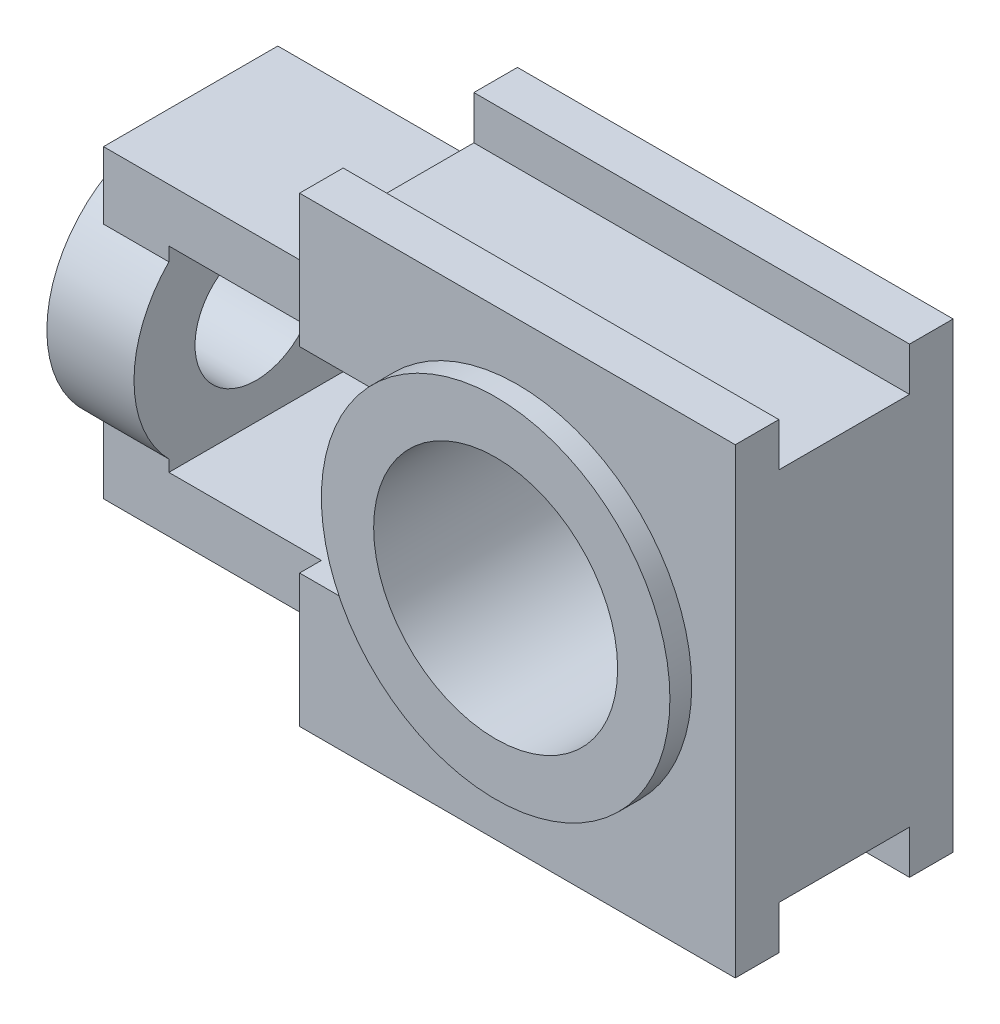
ISO-10303-21;
HEADER;
FILE_DESCRIPTION(('STEP AP214'),'2;1');
FILE_NAME('part.step','',(''),(''),'','','');
FILE_SCHEMA(('AUTOMOTIVE_DESIGN { 1 0 10303 214 1 1 1 1 }'));
ENDSEC;
DATA;
#1=APPLICATION_CONTEXT('core data for automotive mechanical design processes');
#2=APPLICATION_PROTOCOL_DEFINITION('international standard','automotive_design',2000,#1);
#3=PRODUCT_CONTEXT('',#1,'mechanical');
#4=PRODUCT('Part','Part','',(#3));
#5=PRODUCT_RELATED_PRODUCT_CATEGORY('part','',(#4));
#6=PRODUCT_DEFINITION_FORMATION('','',#4);
#7=PRODUCT_DEFINITION_CONTEXT('part definition',#1,'design');
#8=PRODUCT_DEFINITION('design','',#6,#7);
#9=PRODUCT_DEFINITION_SHAPE('','',#8);
#10=(LENGTH_UNIT() NAMED_UNIT(*) SI_UNIT(.MILLI.,.METRE.));
#11=(NAMED_UNIT(*) PLANE_ANGLE_UNIT() SI_UNIT($,.RADIAN.));
#12=(NAMED_UNIT(*) SI_UNIT($,.STERADIAN.) SOLID_ANGLE_UNIT());
#13=UNCERTAINTY_MEASURE_WITH_UNIT(LENGTH_MEASURE(1.E-05),#10,'distance_accuracy_value','');
#14=(GEOMETRIC_REPRESENTATION_CONTEXT(3) GLOBAL_UNCERTAINTY_ASSIGNED_CONTEXT((#13)) GLOBAL_UNIT_ASSIGNED_CONTEXT((#10,
#11,#12)) REPRESENTATION_CONTEXT('',''));
#15=CARTESIAN_POINT('',(0.,0.,0.));
#16=DIRECTION('',(0.,0.,1.));
#17=DIRECTION('',(1.,0.,0.));
#18=AXIS2_PLACEMENT_3D('',#15,#16,#17);
#19=CARTESIAN_POINT('',(-50.,0.,0.));
#20=DIRECTION('',(1.,0.,0.));
#21=DIRECTION('',(0.,0.,-1.));
#22=AXIS2_PLACEMENT_3D('',#19,#20,#21);
#23=PLANE('',#22);
#24=CARTESIAN_POINT('',(-50.,52.75,-25.));
#25=DIRECTION('',(-1.,0.,0.));
#26=DIRECTION('',(0.,0.,1.));
#27=AXIS2_PLACEMENT_3D('',#24,#25,#26);
#28=CIRCLE('',#27,28.);
#29=CARTESIAN_POINT('',(-50.,72.3459179422654,-4.99999999999999));
#30=VERTEX_POINT('',#29);
#31=CARTESIAN_POINT('',(-50.,72.3459179422654,-45.));
#32=VERTEX_POINT('',#31);
#33=EDGE_CURVE('E54',#30,#32,#28,.T.);
#34=ORIENTED_EDGE('',*,*,#33,.F.);
#35=DIRECTION('',(0.,1.,0.));
#36=VECTOR('',#35,1.);
#37=CARTESIAN_POINT('',(-50.,87.75,-5.));
#38=LINE('',#37,#36);
#39=CARTESIAN_POINT('',(-50.,87.75,-5.));
#40=VERTEX_POINT('',#39);
#41=EDGE_CURVE('E332',#30,#40,#38,.T.);
#42=ORIENTED_EDGE('',*,*,#41,.T.);
#43=DIRECTION('',(0.,0.,-1.));
#44=VECTOR('',#43,1.);
#45=CARTESIAN_POINT('',(-50.,87.75,-45.));
#46=LINE('',#45,#44);
#47=CARTESIAN_POINT('',(-50.,87.75,-45.));
#48=VERTEX_POINT('',#47);
#49=EDGE_CURVE('E339',#40,#48,#46,.T.);
#50=ORIENTED_EDGE('',*,*,#49,.T.);
#51=DIRECTION('',(0.,-1.,0.));
#52=VECTOR('',#51,1.);
#53=CARTESIAN_POINT('',(-50.,17.75,-45.));
#54=LINE('',#53,#52);
#55=EDGE_CURVE('E328',#48,#32,#54,.T.);
#56=ORIENTED_EDGE('',*,*,#55,.T.);
#57=EDGE_LOOP('',(#34,#42,#50,#56));
#58=FACE_BOUND('',#57,.T.);
#59=ADVANCED_FACE('F44',(#58),#23,.F.);
#60=CARTESIAN_POINT('',(-50.,33.1540820577346,-45.));
#61=VERTEX_POINT('',#60);
#62=CARTESIAN_POINT('',(-50.,33.1540820577346,-5.));
#63=VERTEX_POINT('',#62);
#64=EDGE_CURVE('E11',#61,#63,#28,.T.);
#65=ORIENTED_EDGE('',*,*,#64,.F.);
#66=CARTESIAN_POINT('',(-50.,17.75,-45.));
#67=VERTEX_POINT('',#66);
#68=EDGE_CURVE('E335',#61,#67,#54,.T.);
#69=ORIENTED_EDGE('',*,*,#68,.T.);
#70=DIRECTION('',(0.,0.,1.));
#71=VECTOR('',#70,1.);
#72=CARTESIAN_POINT('',(-50.,17.75,-5.));
#73=LINE('',#72,#71);
#74=CARTESIAN_POINT('',(-50.,17.75,-5.));
#75=VERTEX_POINT('',#74);
#76=EDGE_CURVE('E331',#67,#75,#73,.T.);
#77=ORIENTED_EDGE('',*,*,#76,.T.);
#78=EDGE_CURVE('E337',#75,#63,#38,.T.);
#79=ORIENTED_EDGE('',*,*,#78,.T.);
#80=EDGE_LOOP('',(#65,#69,#77,#79));
#81=FACE_BOUND('',#80,.T.);
#82=ADVANCED_FACE('F533',(#81),#23,.F.);
#83=CARTESIAN_POINT('',(-50.,87.75,-5.));
#84=DIRECTION('',(0.,0.,-1.));
#85=DIRECTION('',(-1.,0.,0.));
#86=AXIS2_PLACEMENT_3D('',#83,#84,#85);
#87=PLANE('',#86);
#88=DIRECTION('',(1.,0.,0.));
#89=VECTOR('',#88,1.);
#90=CARTESIAN_POINT('',(0.,30.5,-5.));
#91=LINE('',#90,#89);
#92=CARTESIAN_POINT('',(-35.,30.5,-5.));
#93=VERTEX_POINT('',#92);
#94=CARTESIAN_POINT('',(0.,30.5,-5.));
#95=VERTEX_POINT('',#94);
#96=EDGE_CURVE('E323',#93,#95,#91,.T.);
#97=ORIENTED_EDGE('',*,*,#96,.F.);
#98=DIRECTION('',(0.,-1.,0.));
#99=VECTOR('',#98,1.);
#100=CARTESIAN_POINT('',(-35.,75.5,-5.));
#101=LINE('',#100,#99);
#102=CARTESIAN_POINT('',(-35.,33.1540820577346,-5.));
#103=VERTEX_POINT('',#102);
#104=EDGE_CURVE('E294',#103,#93,#101,.T.);
#105=ORIENTED_EDGE('',*,*,#104,.F.);
#106=DIRECTION('',(-1.,0.,0.));
#107=VECTOR('',#106,1.);
#108=CARTESIAN_POINT('',(-35.,33.1540820577346,-5.));
#109=LINE('',#108,#107);
#110=EDGE_CURVE('E325',#103,#63,#109,.T.);
#111=ORIENTED_EDGE('',*,*,#110,.T.);
#112=ORIENTED_EDGE('',*,*,#78,.F.);
#113=DIRECTION('',(1.,0.,0.));
#114=VECTOR('',#113,1.);
#115=CARTESIAN_POINT('',(-50.,17.75,-5.));
#116=LINE('',#115,#114);
#117=CARTESIAN_POINT('',(0.,17.75,-5.));
#118=VERTEX_POINT('',#117);
#119=EDGE_CURVE('E359',#75,#118,#116,.T.);
#120=ORIENTED_EDGE('',*,*,#119,.T.);
#121=DIRECTION('',(0.,1.,0.));
#122=VECTOR('',#121,1.);
#123=CARTESIAN_POINT('',(0.,87.75,-5.));
#124=LINE('',#123,#122);
#125=EDGE_CURVE('E344',#118,#95,#124,.T.);
#126=ORIENTED_EDGE('',*,*,#125,.T.);
#127=EDGE_LOOP('',(#97,#105,#111,#112,#120,#126));
#128=FACE_BOUND('',#127,.T.);
#129=ADVANCED_FACE('F531',(#128),#87,.F.);
#130=CARTESIAN_POINT('',(-50.,75.5,-45.));
#131=DIRECTION('',(0.,0.,1.));
#132=DIRECTION('',(1.,0.,0.));
#133=AXIS2_PLACEMENT_3D('',#130,#131,#132);
#134=PLANE('',#133);
#135=DIRECTION('',(0.,-1.,0.));
#136=VECTOR('',#135,1.);
#137=CARTESIAN_POINT('',(-35.,75.5,-45.));
#138=LINE('',#137,#136);
#139=CARTESIAN_POINT('',(-35.,33.1540820577346,-45.));
#140=VERTEX_POINT('',#139);
#141=CARTESIAN_POINT('',(-35.,30.5,-45.));
#142=VERTEX_POINT('',#141);
#143=EDGE_CURVE('E302',#140,#142,#138,.T.);
#144=ORIENTED_EDGE('',*,*,#143,.T.);
#145=DIRECTION('',(1.,0.,0.));
#146=VECTOR('',#145,1.);
#147=CARTESIAN_POINT('',(-50.,30.5,-45.));
#148=LINE('',#147,#146);
#149=CARTESIAN_POINT('',(0.,30.5,-45.));
#150=VERTEX_POINT('',#149);
#151=EDGE_CURVE('E427',#142,#150,#148,.T.);
#152=ORIENTED_EDGE('',*,*,#151,.T.);
#153=DIRECTION('',(0.,-1.,0.));
#154=VECTOR('',#153,1.);
#155=CARTESIAN_POINT('',(0.,75.5,-45.));
#156=LINE('',#155,#154);
#157=CARTESIAN_POINT('',(0.,17.75,-45.));
#158=VERTEX_POINT('',#157);
#159=EDGE_CURVE('E354',#150,#158,#156,.T.);
#160=ORIENTED_EDGE('',*,*,#159,.T.);
#161=DIRECTION('',(1.,0.,0.));
#162=VECTOR('',#161,1.);
#163=CARTESIAN_POINT('',(-50.,17.75,-45.));
#164=LINE('',#163,#162);
#165=EDGE_CURVE('E361',#67,#158,#164,.T.);
#166=ORIENTED_EDGE('',*,*,#165,.F.);
#167=ORIENTED_EDGE('',*,*,#68,.F.);
#168=DIRECTION('',(-1.,0.,0.));
#169=VECTOR('',#168,1.);
#170=CARTESIAN_POINT('',(-35.,33.1540820577346,-45.));
#171=LINE('',#170,#169);
#172=EDGE_CURVE('E313',#61,#140,#171,.F.);
#173=ORIENTED_EDGE('',*,*,#172,.T.);
#174=EDGE_LOOP('',(#144,#152,#160,#166,#167,#173));
#175=FACE_BOUND('',#174,.T.);
#176=ADVANCED_FACE('F636',(#175),#134,.F.);
#177=CARTESIAN_POINT('',(0.,106.,-50.));
#178=DIRECTION('',(-1.,0.,0.));
#179=DIRECTION('',(0.,0.,1.));
#180=AXIS2_PLACEMENT_3D('',#177,#178,#179);
#181=PLANE('',#180);
#182=DIRECTION('',(0.,0.,-1.));
#183=VECTOR('',#182,1.);
#184=CARTESIAN_POINT('',(0.,87.75,-45.));
#185=LINE('',#184,#183);
#186=CARTESIAN_POINT('',(0.,87.75,-5.));
#187=VERTEX_POINT('',#186);
#188=CARTESIAN_POINT('',(0.,87.75,-45.));
#189=VERTEX_POINT('',#188);
#190=EDGE_CURVE('E350',#187,#189,#185,.T.);
#191=ORIENTED_EDGE('',*,*,#190,.F.);
#192=CARTESIAN_POINT('',(0.,75.5,-5.));
#193=VERTEX_POINT('',#192);
#194=EDGE_CURVE('E343',#193,#187,#124,.T.);
#195=ORIENTED_EDGE('',*,*,#194,.F.);
#196=DIRECTION('',(0.,0.,1.));
#197=VECTOR('',#196,1.);
#198=CARTESIAN_POINT('',(0.,75.5,-50.));
#199=LINE('',#198,#197);
#200=CARTESIAN_POINT('',(0.,75.5,0.));
#201=VERTEX_POINT('',#200);
#202=EDGE_CURVE('E463',#193,#201,#199,.T.);
#203=ORIENTED_EDGE('',*,*,#202,.T.);
#204=DIRECTION('',(0.,-1.,0.));
#205=VECTOR('',#204,1.);
#206=CARTESIAN_POINT('',(0.,106.,0.));
#207=LINE('',#206,#205);
#208=CARTESIAN_POINT('',(0.,106.,0.));
#209=VERTEX_POINT('',#208);
#210=EDGE_CURVE('E481',#209,#201,#207,.T.);
#211=ORIENTED_EDGE('',*,*,#210,.F.);
#212=DIRECTION('',(0.,0.,1.));
#213=VECTOR('',#212,1.);
#214=CARTESIAN_POINT('',(0.,106.,-50.));
#215=LINE('',#214,#213);
#216=CARTESIAN_POINT('',(0.,106.,-10.));
#217=VERTEX_POINT('',#216);
#218=EDGE_CURVE('E480',#217,#209,#215,.T.);
#219=ORIENTED_EDGE('',*,*,#218,.F.);
#220=DIRECTION('',(0.,1.,0.));
#221=VECTOR('',#220,1.);
#222=CARTESIAN_POINT('',(0.,96.,-10.));
#223=LINE('',#222,#221);
#224=CARTESIAN_POINT('',(0.,96.,-10.));
#225=VERTEX_POINT('',#224);
#226=EDGE_CURVE('E399',#225,#217,#223,.T.);
#227=ORIENTED_EDGE('',*,*,#226,.F.);
#228=DIRECTION('',(0.,0.,1.));
#229=VECTOR('',#228,1.);
#230=CARTESIAN_POINT('',(0.,96.,-40.));
#231=LINE('',#230,#229);
#232=CARTESIAN_POINT('',(0.,96.,-40.));
#233=VERTEX_POINT('',#232);
#234=EDGE_CURVE('E403',#233,#225,#231,.T.);
#235=ORIENTED_EDGE('',*,*,#234,.F.);
#236=DIRECTION('',(0.,-1.,0.));
#237=VECTOR('',#236,1.);
#238=CARTESIAN_POINT('',(0.,106.,-40.));
#239=LINE('',#238,#237);
#240=CARTESIAN_POINT('',(0.,106.,-40.));
#241=VERTEX_POINT('',#240);
#242=EDGE_CURVE('E381',#241,#233,#239,.T.);
#243=ORIENTED_EDGE('',*,*,#242,.F.);
#244=CARTESIAN_POINT('',(0.,106.,-50.));
#245=VERTEX_POINT('',#244);
#246=EDGE_CURVE('E473',#245,#241,#215,.T.);
#247=ORIENTED_EDGE('',*,*,#246,.F.);
#248=DIRECTION('',(0.,-1.,0.));
#249=VECTOR('',#248,1.);
#250=CARTESIAN_POINT('',(0.,106.,-50.));
#251=LINE('',#250,#249);
#252=CARTESIAN_POINT('',(0.,75.5,-50.));
#253=VERTEX_POINT('',#252);
#254=EDGE_CURVE('E489',#245,#253,#251,.T.);
#255=ORIENTED_EDGE('',*,*,#254,.T.);
#256=CARTESIAN_POINT('',(0.,75.5,-45.));
#257=VERTEX_POINT('',#256);
#258=EDGE_CURVE('E487',#253,#257,#199,.T.);
#259=ORIENTED_EDGE('',*,*,#258,.T.);
#260=EDGE_CURVE('E351',#189,#257,#156,.T.);
#261=ORIENTED_EDGE('',*,*,#260,.F.);
#262=EDGE_LOOP('',(#191,#195,#203,#211,#219,#227,#235,#243,#247,#255,#259,#261));
#263=FACE_BOUND('',#262,.T.);
#264=ADVANCED_FACE('F50',(#263),#181,.T.);
#265=CARTESIAN_POINT('',(0.,106.,-50.));
#266=DIRECTION('',(-1.,0.,0.));
#267=DIRECTION('',(0.,0.,1.));
#268=AXIS2_PLACEMENT_3D('',#265,#266,#267);
#269=PLANE('',#268);
#270=DIRECTION('',(0.,0.,1.));
#271=VECTOR('',#270,1.);
#272=CARTESIAN_POINT('',(0.,30.5,-50.));
#273=LINE('',#272,#271);
#274=CARTESIAN_POINT('',(0.,30.5,0.));
#275=VERTEX_POINT('',#274);
#276=EDGE_CURVE('E442',#95,#275,#273,.T.);
#277=ORIENTED_EDGE('',*,*,#276,.F.);
#278=ORIENTED_EDGE('',*,*,#125,.F.);
#279=DIRECTION('',(0.,0.,1.));
#280=VECTOR('',#279,1.);
#281=CARTESIAN_POINT('',(0.,17.75,-5.));
#282=LINE('',#281,#280);
#283=EDGE_CURVE('E330',#158,#118,#282,.T.);
#284=ORIENTED_EDGE('',*,*,#283,.F.);
#285=ORIENTED_EDGE('',*,*,#159,.F.);
#286=CARTESIAN_POINT('',(0.,30.5,-50.));
#287=VERTEX_POINT('',#286);
#288=EDGE_CURVE('E447',#287,#150,#273,.T.);
#289=ORIENTED_EDGE('',*,*,#288,.F.);
#290=DIRECTION('',(0.,-1.,0.));
#291=VECTOR('',#290,1.);
#292=CARTESIAN_POINT('',(0.,106.,-50.));
#293=LINE('',#292,#291);
#294=CARTESIAN_POINT('',(0.,0.,-50.));
#295=VERTEX_POINT('',#294);
#296=EDGE_CURVE('E448',#287,#295,#293,.T.);
#297=ORIENTED_EDGE('',*,*,#296,.T.);
#298=DIRECTION('',(0.,0.,1.));
#299=VECTOR('',#298,1.);
#300=CARTESIAN_POINT('',(0.,0.,-50.));
#301=LINE('',#300,#299);
#302=CARTESIAN_POINT('',(0.,0.,-40.));
#303=VERTEX_POINT('',#302);
#304=EDGE_CURVE('E467',#295,#303,#301,.T.);
#305=ORIENTED_EDGE('',*,*,#304,.T.);
#306=DIRECTION('',(0.,-1.,0.));
#307=VECTOR('',#306,1.);
#308=CARTESIAN_POINT('',(0.,10.,-40.));
#309=LINE('',#308,#307);
#310=CARTESIAN_POINT('',(0.,10.,-40.));
#311=VERTEX_POINT('',#310);
#312=EDGE_CURVE('E387',#311,#303,#309,.T.);
#313=ORIENTED_EDGE('',*,*,#312,.F.);
#314=DIRECTION('',(0.,0.,-1.));
#315=VECTOR('',#314,1.);
#316=CARTESIAN_POINT('',(0.,10.,-10.));
#317=LINE('',#316,#315);
#318=CARTESIAN_POINT('',(0.,9.99999999999999,-10.));
#319=VERTEX_POINT('',#318);
#320=EDGE_CURVE('E367',#319,#311,#317,.T.);
#321=ORIENTED_EDGE('',*,*,#320,.F.);
#322=DIRECTION('',(0.,-1.,0.));
#323=VECTOR('',#322,1.);
#324=CARTESIAN_POINT('',(0.,10.,-10.));
#325=LINE('',#324,#323);
#326=CARTESIAN_POINT('',(0.,0.,-10.));
#327=VERTEX_POINT('',#326);
#328=EDGE_CURVE('E378',#319,#327,#325,.T.);
#329=ORIENTED_EDGE('',*,*,#328,.T.);
#330=CARTESIAN_POINT('',(0.,0.,0.));
#331=VERTEX_POINT('',#330);
#332=EDGE_CURVE('E459',#327,#331,#301,.T.);
#333=ORIENTED_EDGE('',*,*,#332,.T.);
#334=DIRECTION('',(0.,-1.,0.));
#335=VECTOR('',#334,1.);
#336=CARTESIAN_POINT('',(0.,106.,0.));
#337=LINE('',#336,#335);
#338=EDGE_CURVE('E446',#275,#331,#337,.T.);
#339=ORIENTED_EDGE('',*,*,#338,.F.);
#340=EDGE_LOOP('',(#277,#278,#284,#285,#289,#297,#305,#313,#321,#329,#333,#339));
#341=FACE_BOUND('',#340,.T.);
#342=ADVANCED_FACE('F549',(#341),#269,.T.);
#343=CARTESIAN_POINT('',(0.,0.,-50.));
#344=DIRECTION('',(0.,-1.,0.));
#345=DIRECTION('',(0.,0.,-1.));
#346=AXIS2_PLACEMENT_3D('',#343,#344,#345);
#347=PLANE('',#346);
#348=DIRECTION('',(-1.,0.,0.));
#349=VECTOR('',#348,1.);
#350=CARTESIAN_POINT('',(0.,0.,-10.));
#351=LINE('',#350,#349);
#352=CARTESIAN_POINT('',(100.,0.,-10.));
#353=VERTEX_POINT('',#352);
#354=EDGE_CURVE('E366',#353,#327,#351,.T.);
#355=ORIENTED_EDGE('',*,*,#354,.F.);
#356=DIRECTION('',(0.,0.,1.));
#357=VECTOR('',#356,1.);
#358=CARTESIAN_POINT('',(100.,0.,-50.));
#359=LINE('',#358,#357);
#360=CARTESIAN_POINT('',(100.,0.,0.));
#361=VERTEX_POINT('',#360);
#362=EDGE_CURVE('E462',#353,#361,#359,.T.);
#363=ORIENTED_EDGE('',*,*,#362,.T.);
#364=DIRECTION('',(1.,0.,0.));
#365=VECTOR('',#364,1.);
#366=CARTESIAN_POINT('',(0.,0.,0.));
#367=LINE('',#366,#365);
#368=EDGE_CURVE('E452',#331,#361,#367,.T.);
#369=ORIENTED_EDGE('',*,*,#368,.F.);
#370=ORIENTED_EDGE('',*,*,#332,.F.);
#371=EDGE_LOOP('',(#355,#363,#369,#370));
#372=FACE_BOUND('',#371,.T.);
#373=ADVANCED_FACE('F589',(#372),#347,.T.);
#374=CARTESIAN_POINT('',(100.,106.,-50.));
#375=DIRECTION('',(0.,1.,0.));
#376=DIRECTION('',(0.,0.,1.));
#377=AXIS2_PLACEMENT_3D('',#374,#375,#376);
#378=PLANE('',#377);
#379=DIRECTION('',(-1.,0.,0.));
#380=VECTOR('',#379,1.);
#381=CARTESIAN_POINT('',(100.,106.,-40.));
#382=LINE('',#381,#380);
#383=CARTESIAN_POINT('',(100.,106.,-40.));
#384=VERTEX_POINT('',#383);
#385=EDGE_CURVE('E408',#384,#241,#382,.T.);
#386=ORIENTED_EDGE('',*,*,#385,.F.);
#387=DIRECTION('',(0.,0.,1.));
#388=VECTOR('',#387,1.);
#389=CARTESIAN_POINT('',(100.,106.,-50.));
#390=LINE('',#389,#388);
#391=CARTESIAN_POINT('',(100.,106.,-50.));
#392=VERTEX_POINT('',#391);
#393=EDGE_CURVE('E469',#392,#384,#390,.T.);
#394=ORIENTED_EDGE('',*,*,#393,.F.);
#395=DIRECTION('',(-1.,0.,0.));
#396=VECTOR('',#395,1.);
#397=CARTESIAN_POINT('',(100.,106.,-50.));
#398=LINE('',#397,#396);
#399=EDGE_CURVE('E483',#392,#245,#398,.T.);
#400=ORIENTED_EDGE('',*,*,#399,.T.);
#401=ORIENTED_EDGE('',*,*,#246,.T.);
#402=EDGE_LOOP('',(#386,#394,#400,#401));
#403=FACE_BOUND('',#402,.T.);
#404=ADVANCED_FACE('F601',(#403),#378,.T.);
#405=CARTESIAN_POINT('',(100.,0.,-50.));
#406=DIRECTION('',(1.,0.,0.));
#407=DIRECTION('',(0.,0.,-1.));
#408=AXIS2_PLACEMENT_3D('',#405,#406,#407);
#409=PLANE('',#408);
#410=DIRECTION('',(0.,-1.,0.));
#411=VECTOR('',#410,1.);
#412=CARTESIAN_POINT('',(100.,10.,-10.));
#413=LINE('',#412,#411);
#414=CARTESIAN_POINT('',(100.,10.,-10.));
#415=VERTEX_POINT('',#414);
#416=EDGE_CURVE('E385',#415,#353,#413,.T.);
#417=ORIENTED_EDGE('',*,*,#416,.F.);
#418=DIRECTION('',(0.,0.,1.));
#419=VECTOR('',#418,1.);
#420=CARTESIAN_POINT('',(100.,10.,-10.));
#421=LINE('',#420,#419);
#422=CARTESIAN_POINT('',(100.,10.,-40.));
#423=VERTEX_POINT('',#422);
#424=EDGE_CURVE('E376',#423,#415,#421,.T.);
#425=ORIENTED_EDGE('',*,*,#424,.F.);
#426=DIRECTION('',(0.,-1.,0.));
#427=VECTOR('',#426,1.);
#428=CARTESIAN_POINT('',(100.,10.,-40.));
#429=LINE('',#428,#427);
#430=CARTESIAN_POINT('',(100.,0.,-40.));
#431=VERTEX_POINT('',#430);
#432=EDGE_CURVE('E383',#423,#431,#429,.T.);
#433=ORIENTED_EDGE('',*,*,#432,.T.);
#434=CARTESIAN_POINT('',(100.,0.,-50.));
#435=VERTEX_POINT('',#434);
#436=EDGE_CURVE('E464',#435,#431,#359,.T.);
#437=ORIENTED_EDGE('',*,*,#436,.F.);
#438=DIRECTION('',(0.,1.,0.));
#439=VECTOR('',#438,1.);
#440=CARTESIAN_POINT('',(100.,0.,-50.));
#441=LINE('',#440,#439);
#442=EDGE_CURVE('E494',#435,#392,#441,.T.);
#443=ORIENTED_EDGE('',*,*,#442,.T.);
#444=ORIENTED_EDGE('',*,*,#393,.T.);
#445=DIRECTION('',(0.,-1.,0.));
#446=VECTOR('',#445,1.);
#447=CARTESIAN_POINT('',(100.,106.,-40.));
#448=LINE('',#447,#446);
#449=CARTESIAN_POINT('',(100.,96.,-40.));
#450=VERTEX_POINT('',#449);
#451=EDGE_CURVE('E391',#384,#450,#448,.T.);
#452=ORIENTED_EDGE('',*,*,#451,.T.);
#453=DIRECTION('',(0.,0.,1.));
#454=VECTOR('',#453,1.);
#455=CARTESIAN_POINT('',(100.,96.,-40.));
#456=LINE('',#455,#454);
#457=CARTESIAN_POINT('',(100.,96.,-10.));
#458=VERTEX_POINT('',#457);
#459=EDGE_CURVE('E392',#450,#458,#456,.T.);
#460=ORIENTED_EDGE('',*,*,#459,.T.);
#461=DIRECTION('',(0.,1.,0.));
#462=VECTOR('',#461,1.);
#463=CARTESIAN_POINT('',(100.,96.,-10.));
#464=LINE('',#463,#462);
#465=CARTESIAN_POINT('',(100.,106.,-10.));
#466=VERTEX_POINT('',#465);
#467=EDGE_CURVE('E398',#458,#466,#464,.T.);
#468=ORIENTED_EDGE('',*,*,#467,.T.);
#469=CARTESIAN_POINT('',(100.,106.,0.));
#470=VERTEX_POINT('',#469);
#471=EDGE_CURVE('E472',#466,#470,#390,.T.);
#472=ORIENTED_EDGE('',*,*,#471,.T.);
#473=DIRECTION('',(0.,1.,0.));
#474=VECTOR('',#473,1.);
#475=CARTESIAN_POINT('',(100.,0.,0.));
#476=LINE('',#475,#474);
#477=EDGE_CURVE('E485',#361,#470,#476,.T.);
#478=ORIENTED_EDGE('',*,*,#477,.F.);
#479=ORIENTED_EDGE('',*,*,#362,.F.);
#480=EDGE_LOOP('',(#417,#425,#433,#437,#443,#444,#452,#460,#468,#472,#478,#479));
#481=FACE_BOUND('',#480,.T.);
#482=ADVANCED_FACE('F577',(#481),#409,.T.);
#483=CARTESIAN_POINT('',(0.,0.,-50.));
#484=DIRECTION('',(0.,0.,1.));
#485=DIRECTION('',(1.,0.,0.));
#486=AXIS2_PLACEMENT_3D('',#483,#484,#485);
#487=PLANE('',#486);
#488=DIRECTION('',(1.,0.,0.));
#489=VECTOR('',#488,1.);
#490=CARTESIAN_POINT('',(100.,30.5,-50.));
#491=LINE('',#490,#489);
#492=CARTESIAN_POINT('',(16.9281086116926,30.5,-50.));
#493=VERTEX_POINT('',#492);
#494=EDGE_CURVE('E439',#287,#493,#491,.T.);
#495=ORIENTED_EDGE('',*,*,#494,.T.);
#496=CARTESIAN_POINT('',(50.,53.,-50.));
#497=DIRECTION('',(0.,0.,1.));
#498=DIRECTION('',(1.,0.,0.));
#499=AXIS2_PLACEMENT_3D('',#496,#497,#498);
#500=CIRCLE('',#499,40.);
#501=CARTESIAN_POINT('',(16.9281086116926,75.5,-50.));
#502=VERTEX_POINT('',#501);
#503=EDGE_CURVE('E432',#493,#502,#500,.T.);
#504=ORIENTED_EDGE('',*,*,#503,.T.);
#505=DIRECTION('',(-1.,0.,0.));
#506=VECTOR('',#505,1.);
#507=CARTESIAN_POINT('',(0.,75.5,-50.));
#508=LINE('',#507,#506);
#509=EDGE_CURVE('E475',#502,#253,#508,.T.);
#510=ORIENTED_EDGE('',*,*,#509,.T.);
#511=ORIENTED_EDGE('',*,*,#254,.F.);
#512=ORIENTED_EDGE('',*,*,#399,.F.);
#513=ORIENTED_EDGE('',*,*,#442,.F.);
#514=DIRECTION('',(1.,0.,0.));
#515=VECTOR('',#514,1.);
#516=CARTESIAN_POINT('',(0.,0.,-50.));
#517=LINE('',#516,#515);
#518=EDGE_CURVE('E455',#295,#435,#517,.T.);
#519=ORIENTED_EDGE('',*,*,#518,.F.);
#520=ORIENTED_EDGE('',*,*,#296,.F.);
#521=EDGE_LOOP('',(#495,#504,#510,#511,#512,#513,#519,#520));
#522=FACE_BOUND('',#521,.T.);
#523=ADVANCED_FACE('F563',(#522),#487,.F.);
#524=CARTESIAN_POINT('',(0.,0.,0.));
#525=DIRECTION('',(0.,0.,1.));
#526=DIRECTION('',(1.,0.,0.));
#527=AXIS2_PLACEMENT_3D('',#524,#525,#526);
#528=PLANE('',#527);
#529=CARTESIAN_POINT('',(50.,53.,0.));
#530=DIRECTION('',(0.,0.,1.));
#531=DIRECTION('',(1.,0.,0.));
#532=AXIS2_PLACEMENT_3D('',#529,#530,#531);
#533=CIRCLE('',#532,40.);
#534=CARTESIAN_POINT('',(16.9281086116926,30.5,0.));
#535=VERTEX_POINT('',#534);
#536=CARTESIAN_POINT('',(16.9281086116926,75.5,0.));
#537=VERTEX_POINT('',#536);
#538=EDGE_CURVE('E430',#535,#537,#533,.T.);
#539=ORIENTED_EDGE('',*,*,#538,.F.);
#540=DIRECTION('',(1.,0.,0.));
#541=VECTOR('',#540,1.);
#542=CARTESIAN_POINT('',(100.,30.5,0.));
#543=LINE('',#542,#541);
#544=EDGE_CURVE('E437',#275,#535,#543,.T.);
#545=ORIENTED_EDGE('',*,*,#544,.F.);
#546=ORIENTED_EDGE('',*,*,#338,.T.);
#547=ORIENTED_EDGE('',*,*,#368,.T.);
#548=ORIENTED_EDGE('',*,*,#477,.T.);
#549=DIRECTION('',(-1.,0.,0.));
#550=VECTOR('',#549,1.);
#551=CARTESIAN_POINT('',(100.,106.,0.));
#552=LINE('',#551,#550);
#553=EDGE_CURVE('E478',#470,#209,#552,.T.);
#554=ORIENTED_EDGE('',*,*,#553,.T.);
#555=ORIENTED_EDGE('',*,*,#210,.T.);
#556=DIRECTION('',(-1.,0.,0.));
#557=VECTOR('',#556,1.);
#558=CARTESIAN_POINT('',(0.,75.5,0.));
#559=LINE('',#558,#557);
#560=EDGE_CURVE('E476',#537,#201,#559,.T.);
#561=ORIENTED_EDGE('',*,*,#560,.F.);
#562=EDGE_LOOP('',(#539,#545,#546,#547,#548,#554,#555,#561));
#563=FACE_BOUND('',#562,.T.);
#564=ADVANCED_FACE('F551',(#563),#528,.T.);
#565=DIRECTION('',(-1.,0.,0.));
#566=VECTOR('',#565,1.);
#567=CARTESIAN_POINT('',(100.,106.,-10.));
#568=LINE('',#567,#566);
#569=EDGE_CURVE('E411',#466,#217,#568,.T.);
#570=ORIENTED_EDGE('',*,*,#569,.T.);
#571=ORIENTED_EDGE('',*,*,#218,.T.);
#572=ORIENTED_EDGE('',*,*,#553,.F.);
#573=ORIENTED_EDGE('',*,*,#471,.F.);
#574=EDGE_LOOP('',(#570,#571,#572,#573));
#575=FACE_BOUND('',#574,.T.);
#576=ADVANCED_FACE('F594',(#575),#378,.T.);
#577=CARTESIAN_POINT('',(0.,75.5,-50.));
#578=DIRECTION('',(0.,1.,0.));
#579=DIRECTION('',(0.,0.,1.));
#580=AXIS2_PLACEMENT_3D('',#577,#578,#579);
#581=PLANE('',#580);
#582=ORIENTED_EDGE('',*,*,#509,.F.);
#583=DIRECTION('',(0.,0.,1.));
#584=VECTOR('',#583,1.);
#585=CARTESIAN_POINT('',(16.9281086116926,75.5,-55.));
#586=LINE('',#585,#584);
#587=EDGE_CURVE('E436',#502,#537,#586,.T.);
#588=ORIENTED_EDGE('',*,*,#587,.T.);
#589=ORIENTED_EDGE('',*,*,#560,.T.);
#590=ORIENTED_EDGE('',*,*,#202,.F.);
#591=DIRECTION('',(-1.,0.,0.));
#592=VECTOR('',#591,1.);
#593=CARTESIAN_POINT('',(-30.,75.5,-5.));
#594=LINE('',#593,#592);
#595=CARTESIAN_POINT('',(-35.,75.5,-5.));
#596=VERTEX_POINT('',#595);
#597=EDGE_CURVE('E329',#193,#596,#594,.T.);
#598=ORIENTED_EDGE('',*,*,#597,.T.);
#599=DIRECTION('',(0.,0.,1.));
#600=VECTOR('',#599,1.);
#601=CARTESIAN_POINT('',(-35.,75.5,-55.));
#602=LINE('',#601,#600);
#603=CARTESIAN_POINT('',(-35.,75.5,-45.));
#604=VERTEX_POINT('',#603);
#605=EDGE_CURVE('E297',#604,#596,#602,.T.);
#606=ORIENTED_EDGE('',*,*,#605,.F.);
#607=DIRECTION('',(-1.,0.,0.));
#608=VECTOR('',#607,1.);
#609=CARTESIAN_POINT('',(-50.,75.5,-45.));
#610=LINE('',#609,#608);
#611=EDGE_CURVE('E47',#257,#604,#610,.T.);
#612=ORIENTED_EDGE('',*,*,#611,.F.);
#613=ORIENTED_EDGE('',*,*,#258,.F.);
#614=EDGE_LOOP('',(#582,#588,#589,#590,#598,#606,#612,#613));
#615=FACE_BOUND('',#614,.T.);
#616=ADVANCED_FACE('F516',(#615),#581,.F.);
#617=DIRECTION('',(1.,0.,0.));
#618=VECTOR('',#617,1.);
#619=CARTESIAN_POINT('',(100.,0.,-40.));
#620=LINE('',#619,#618);
#621=EDGE_CURVE('E369',#303,#431,#620,.T.);
#622=ORIENTED_EDGE('',*,*,#621,.F.);
#623=ORIENTED_EDGE('',*,*,#304,.F.);
#624=ORIENTED_EDGE('',*,*,#518,.T.);
#625=ORIENTED_EDGE('',*,*,#436,.T.);
#626=EDGE_LOOP('',(#622,#623,#624,#625));
#627=FACE_BOUND('',#626,.T.);
#628=ADVANCED_FACE('F567',(#627),#347,.T.);
#629=CARTESIAN_POINT('',(100.,30.5,-50.));
#630=DIRECTION('',(0.,-1.,0.));
#631=DIRECTION('',(0.,0.,-1.));
#632=AXIS2_PLACEMENT_3D('',#629,#630,#631);
#633=PLANE('',#632);
#634=ORIENTED_EDGE('',*,*,#544,.T.);
#635=DIRECTION('',(0.,0.,1.));
#636=VECTOR('',#635,1.);
#637=CARTESIAN_POINT('',(16.9281086116926,30.5,-55.));
#638=LINE('',#637,#636);
#639=EDGE_CURVE('E431',#535,#493,#638,.F.);
#640=ORIENTED_EDGE('',*,*,#639,.T.);
#641=ORIENTED_EDGE('',*,*,#494,.F.);
#642=ORIENTED_EDGE('',*,*,#288,.T.);
#643=ORIENTED_EDGE('',*,*,#151,.F.);
#644=DIRECTION('',(0.,0.,1.));
#645=VECTOR('',#644,1.);
#646=CARTESIAN_POINT('',(-35.,30.5,-55.));
#647=LINE('',#646,#645);
#648=EDGE_CURVE('E301',#142,#93,#647,.T.);
#649=ORIENTED_EDGE('',*,*,#648,.T.);
#650=ORIENTED_EDGE('',*,*,#96,.T.);
#651=ORIENTED_EDGE('',*,*,#276,.T.);
#652=EDGE_LOOP('',(#634,#640,#641,#642,#643,#649,#650,#651));
#653=FACE_BOUND('',#652,.T.);
#654=ADVANCED_FACE('F547',(#653),#633,.F.);
#655=CARTESIAN_POINT('',(50.,53.,-55.));
#656=DIRECTION('',(0.,0.,1.));
#657=DIRECTION('',(1.,0.,0.));
#658=AXIS2_PLACEMENT_3D('',#655,#656,#657);
#659=CYLINDRICAL_SURFACE('',#658,40.);
#660=CARTESIAN_POINT('',(50.,53.,-55.));
#661=DIRECTION('',(0.,0.,1.));
#662=DIRECTION('',(1.,0.,0.));
#663=AXIS2_PLACEMENT_3D('',#660,#661,#662);
#664=CIRCLE('',#663,40.);
#665=CARTESIAN_POINT('',(90.,53.,-55.));
#666=VERTEX_POINT('',#665);
#667=EDGE_CURVE('E428',#666,#666,#664,.T.);
#668=ORIENTED_EDGE('',*,*,#667,.T.);
#669=EDGE_LOOP('',(#668));
#670=FACE_BOUND('',#669,.T.);
#671=ORIENTED_EDGE('',*,*,#587,.F.);
#672=ORIENTED_EDGE('',*,*,#503,.F.);
#673=ORIENTED_EDGE('',*,*,#639,.F.);
#674=ORIENTED_EDGE('',*,*,#538,.T.);
#675=EDGE_LOOP('',(#671,#672,#673,#674));
#676=FACE_BOUND('',#675,.T.);
#677=CARTESIAN_POINT('',(50.,53.,5.));
#678=DIRECTION('',(0.,0.,1.));
#679=DIRECTION('',(1.,0.,0.));
#680=AXIS2_PLACEMENT_3D('',#677,#678,#679);
#681=CIRCLE('',#680,40.);
#682=CARTESIAN_POINT('',(90.,53.,5.));
#683=VERTEX_POINT('',#682);
#684=EDGE_CURVE('E423',#683,#683,#681,.T.);
#685=ORIENTED_EDGE('',*,*,#684,.F.);
#686=EDGE_LOOP('',(#685));
#687=FACE_BOUND('',#686,.T.);
#688=ADVANCED_FACE('F560',(#670,#676,#687),#659,.T.);
#689=CARTESIAN_POINT('',(50.,53.,-55.));
#690=DIRECTION('',(0.,0.,1.));
#691=DIRECTION('',(1.,0.,0.));
#692=AXIS2_PLACEMENT_3D('',#689,#690,#691);
#693=PLANE('',#692);
#694=CARTESIAN_POINT('',(50.,53.,-55.));
#695=DIRECTION('',(0.,0.,1.));
#696=DIRECTION('',(1.,0.,0.));
#697=AXIS2_PLACEMENT_3D('',#694,#695,#696);
#698=CIRCLE('',#697,28.);
#699=CARTESIAN_POINT('',(78.,53.,-55.));
#700=VERTEX_POINT('',#699);
#701=EDGE_CURVE('E420',#700,#700,#698,.T.);
#702=ORIENTED_EDGE('',*,*,#701,.T.);
#703=EDGE_LOOP('',(#702));
#704=FACE_BOUND('',#703,.T.);
#705=ORIENTED_EDGE('',*,*,#667,.F.);
#706=EDGE_LOOP('',(#705));
#707=FACE_BOUND('',#706,.T.);
#708=ADVANCED_FACE('F930',(#704,#707),#693,.F.);
#709=CARTESIAN_POINT('',(50.,53.,5.));
#710=DIRECTION('',(0.,0.,1.));
#711=DIRECTION('',(1.,0.,0.));
#712=AXIS2_PLACEMENT_3D('',#709,#710,#711);
#713=PLANE('',#712);
#714=CARTESIAN_POINT('',(50.,53.,5.));
#715=DIRECTION('',(0.,0.,1.));
#716=DIRECTION('',(1.,0.,0.));
#717=AXIS2_PLACEMENT_3D('',#714,#715,#716);
#718=CIRCLE('',#717,28.);
#719=CARTESIAN_POINT('',(78.,53.,5.));
#720=VERTEX_POINT('',#719);
#721=EDGE_CURVE('E414',#720,#720,#718,.T.);
#722=ORIENTED_EDGE('',*,*,#721,.F.);
#723=EDGE_LOOP('',(#722));
#724=FACE_BOUND('',#723,.T.);
#725=ORIENTED_EDGE('',*,*,#684,.T.);
#726=EDGE_LOOP('',(#725));
#727=FACE_BOUND('',#726,.T.);
#728=ADVANCED_FACE('F912',(#724,#727),#713,.T.);
#729=CARTESIAN_POINT('',(50.,53.,-55.));
#730=DIRECTION('',(0.,0.,1.));
#731=DIRECTION('',(1.,0.,0.));
#732=AXIS2_PLACEMENT_3D('',#729,#730,#731);
#733=CYLINDRICAL_SURFACE('',#732,28.);
#734=ORIENTED_EDGE('',*,*,#701,.F.);
#735=EDGE_LOOP('',(#734));
#736=FACE_BOUND('',#735,.T.);
#737=ORIENTED_EDGE('',*,*,#721,.T.);
#738=EDGE_LOOP('',(#737));
#739=FACE_BOUND('',#738,.T.);
#740=ADVANCED_FACE('F619',(#736,#739),#733,.F.);
#741=CARTESIAN_POINT('',(100.,106.,-40.));
#742=DIRECTION('',(0.,0.,-1.));
#743=DIRECTION('',(-1.,0.,0.));
#744=AXIS2_PLACEMENT_3D('',#741,#742,#743);
#745=PLANE('',#744);
#746=ORIENTED_EDGE('',*,*,#242,.T.);
#747=DIRECTION('',(-1.,0.,0.));
#748=VECTOR('',#747,1.);
#749=CARTESIAN_POINT('',(100.,96.,-40.));
#750=LINE('',#749,#748);
#751=EDGE_CURVE('E405',#450,#233,#750,.T.);
#752=ORIENTED_EDGE('',*,*,#751,.F.);
#753=ORIENTED_EDGE('',*,*,#451,.F.);
#754=ORIENTED_EDGE('',*,*,#385,.T.);
#755=EDGE_LOOP('',(#746,#752,#753,#754));
#756=FACE_BOUND('',#755,.T.);
#757=ADVANCED_FACE('F603',(#756),#745,.F.);
#758=CARTESIAN_POINT('',(100.,96.,-10.));
#759=DIRECTION('',(0.,0.,1.));
#760=DIRECTION('',(1.,0.,0.));
#761=AXIS2_PLACEMENT_3D('',#758,#759,#760);
#762=PLANE('',#761);
#763=ORIENTED_EDGE('',*,*,#226,.T.);
#764=ORIENTED_EDGE('',*,*,#569,.F.);
#765=ORIENTED_EDGE('',*,*,#467,.F.);
#766=DIRECTION('',(-1.,0.,0.));
#767=VECTOR('',#766,1.);
#768=CARTESIAN_POINT('',(100.,96.,-10.));
#769=LINE('',#768,#767);
#770=EDGE_CURVE('E412',#458,#225,#769,.T.);
#771=ORIENTED_EDGE('',*,*,#770,.T.);
#772=EDGE_LOOP('',(#763,#764,#765,#771));
#773=FACE_BOUND('',#772,.T.);
#774=ADVANCED_FACE('F614',(#773),#762,.F.);
#775=CARTESIAN_POINT('',(100.,96.,-40.));
#776=DIRECTION('',(0.,-1.,0.));
#777=DIRECTION('',(0.,0.,-1.));
#778=AXIS2_PLACEMENT_3D('',#775,#776,#777);
#779=PLANE('',#778);
#780=ORIENTED_EDGE('',*,*,#234,.T.);
#781=ORIENTED_EDGE('',*,*,#770,.F.);
#782=ORIENTED_EDGE('',*,*,#459,.F.);
#783=ORIENTED_EDGE('',*,*,#751,.T.);
#784=EDGE_LOOP('',(#780,#781,#782,#783));
#785=FACE_BOUND('',#784,.T.);
#786=ADVANCED_FACE('F610',(#785),#779,.F.);
#787=CARTESIAN_POINT('',(0.,10.,-10.));
#788=DIRECTION('',(0.,0.,1.));
#789=DIRECTION('',(1.,0.,0.));
#790=AXIS2_PLACEMENT_3D('',#787,#788,#789);
#791=PLANE('',#790);
#792=ORIENTED_EDGE('',*,*,#354,.T.);
#793=ORIENTED_EDGE('',*,*,#328,.F.);
#794=DIRECTION('',(-1.,0.,0.));
#795=VECTOR('',#794,1.);
#796=CARTESIAN_POINT('',(0.,10.,-10.));
#797=LINE('',#796,#795);
#798=EDGE_CURVE('E370',#415,#319,#797,.T.);
#799=ORIENTED_EDGE('',*,*,#798,.F.);
#800=ORIENTED_EDGE('',*,*,#416,.T.);
#801=EDGE_LOOP('',(#792,#793,#799,#800));
#802=FACE_BOUND('',#801,.T.);
#803=ADVANCED_FACE('F616',(#802),#791,.F.);
#804=CARTESIAN_POINT('',(100.,10.,-40.));
#805=DIRECTION('',(0.,0.,-1.));
#806=DIRECTION('',(-1.,0.,0.));
#807=AXIS2_PLACEMENT_3D('',#804,#805,#806);
#808=PLANE('',#807);
#809=ORIENTED_EDGE('',*,*,#621,.T.);
#810=ORIENTED_EDGE('',*,*,#432,.F.);
#811=DIRECTION('',(1.,0.,0.));
#812=VECTOR('',#811,1.);
#813=CARTESIAN_POINT('',(100.,10.,-40.));
#814=LINE('',#813,#812);
#815=EDGE_CURVE('E373',#311,#423,#814,.T.);
#816=ORIENTED_EDGE('',*,*,#815,.F.);
#817=ORIENTED_EDGE('',*,*,#312,.T.);
#818=EDGE_LOOP('',(#809,#810,#816,#817));
#819=FACE_BOUND('',#818,.T.);
#820=ADVANCED_FACE('F575',(#819),#808,.F.);
#821=CARTESIAN_POINT('',(0.,10.,0.));
#822=DIRECTION('',(0.,1.,0.));
#823=DIRECTION('',(0.,0.,1.));
#824=AXIS2_PLACEMENT_3D('',#821,#822,#823);
#825=PLANE('',#824);
#826=ORIENTED_EDGE('',*,*,#798,.T.);
#827=ORIENTED_EDGE('',*,*,#320,.T.);
#828=ORIENTED_EDGE('',*,*,#815,.T.);
#829=ORIENTED_EDGE('',*,*,#424,.T.);
#830=EDGE_LOOP('',(#826,#827,#828,#829));
#831=FACE_BOUND('',#830,.T.);
#832=ADVANCED_FACE('F576',(#831),#825,.F.);
#833=CARTESIAN_POINT('',(-50.,17.75,-5.));
#834=DIRECTION('',(0.,1.,0.));
#835=DIRECTION('',(0.,0.,1.));
#836=AXIS2_PLACEMENT_3D('',#833,#834,#835);
#837=PLANE('',#836);
#838=ORIENTED_EDGE('',*,*,#283,.T.);
#839=ORIENTED_EDGE('',*,*,#119,.F.);
#840=ORIENTED_EDGE('',*,*,#76,.F.);
#841=ORIENTED_EDGE('',*,*,#165,.T.);
#842=EDGE_LOOP('',(#838,#839,#840,#841));
#843=FACE_BOUND('',#842,.T.);
#844=ADVANCED_FACE('F544',(#843),#837,.F.);
#845=DIRECTION('',(-1.,0.,0.));
#846=VECTOR('',#845,1.);
#847=CARTESIAN_POINT('',(-35.,72.3459179422654,-5.));
#848=LINE('',#847,#846);
#849=CARTESIAN_POINT('',(-35.,72.3459179422654,-5.));
#850=VERTEX_POINT('',#849);
#851=EDGE_CURVE('E316',#30,#850,#848,.F.);
#852=ORIENTED_EDGE('',*,*,#851,.T.);
#853=EDGE_CURVE('E296',#596,#850,#101,.T.);
#854=ORIENTED_EDGE('',*,*,#853,.F.);
#855=ORIENTED_EDGE('',*,*,#597,.F.);
#856=ORIENTED_EDGE('',*,*,#194,.T.);
#857=DIRECTION('',(1.,0.,0.));
#858=VECTOR('',#857,1.);
#859=CARTESIAN_POINT('',(-50.,87.75,-5.));
#860=LINE('',#859,#858);
#861=EDGE_CURVE('E357',#40,#187,#860,.T.);
#862=ORIENTED_EDGE('',*,*,#861,.F.);
#863=ORIENTED_EDGE('',*,*,#41,.F.);
#864=EDGE_LOOP('',(#852,#854,#855,#856,#862,#863));
#865=FACE_BOUND('',#864,.T.);
#866=ADVANCED_FACE('F524',(#865),#87,.F.);
#867=CARTESIAN_POINT('',(-50.,87.75,-45.));
#868=DIRECTION('',(0.,-1.,0.));
#869=DIRECTION('',(0.,0.,-1.));
#870=AXIS2_PLACEMENT_3D('',#867,#868,#869);
#871=PLANE('',#870);
#872=ORIENTED_EDGE('',*,*,#190,.T.);
#873=DIRECTION('',(1.,0.,0.));
#874=VECTOR('',#873,1.);
#875=CARTESIAN_POINT('',(-50.,87.75,-45.));
#876=LINE('',#875,#874);
#877=EDGE_CURVE('E345',#48,#189,#876,.T.);
#878=ORIENTED_EDGE('',*,*,#877,.F.);
#879=ORIENTED_EDGE('',*,*,#49,.F.);
#880=ORIENTED_EDGE('',*,*,#861,.T.);
#881=EDGE_LOOP('',(#872,#878,#879,#880));
#882=FACE_BOUND('',#881,.T.);
#883=ADVANCED_FACE('F634',(#882),#871,.F.);
#884=ORIENTED_EDGE('',*,*,#611,.T.);
#885=CARTESIAN_POINT('',(-35.,72.3459179422654,-45.));
#886=VERTEX_POINT('',#885);
#887=EDGE_CURVE('E307',#604,#886,#138,.T.);
#888=ORIENTED_EDGE('',*,*,#887,.T.);
#889=DIRECTION('',(-1.,0.,0.));
#890=VECTOR('',#889,1.);
#891=CARTESIAN_POINT('',(-35.,72.3459179422654,-45.));
#892=LINE('',#891,#890);
#893=EDGE_CURVE('E320',#886,#32,#892,.T.);
#894=ORIENTED_EDGE('',*,*,#893,.T.);
#895=ORIENTED_EDGE('',*,*,#55,.F.);
#896=ORIENTED_EDGE('',*,*,#877,.T.);
#897=ORIENTED_EDGE('',*,*,#260,.T.);
#898=EDGE_LOOP('',(#884,#888,#894,#895,#896,#897));
#899=FACE_BOUND('',#898,.T.);
#900=ADVANCED_FACE('F506',(#899),#134,.F.);
#901=CARTESIAN_POINT('',(-35.,52.75,-25.));
#902=DIRECTION('',(-1.,0.,0.));
#903=DIRECTION('',(0.,0.,1.));
#904=AXIS2_PLACEMENT_3D('',#901,#902,#903);
#905=PLANE('',#904);
#906=CARTESIAN_POINT('',(-35.,52.75,-25.));
#907=DIRECTION('',(-1.,0.,0.));
#908=DIRECTION('',(0.,0.,1.));
#909=AXIS2_PLACEMENT_3D('',#906,#907,#908);
#910=CIRCLE('',#909,14.);
#911=CARTESIAN_POINT('',(-35.,64.8743556529821,-32.));
#912=VERTEX_POINT('',#911);
#913=CARTESIAN_POINT('',(-35.,64.8743556529821,-18.));
#914=VERTEX_POINT('',#913);
#915=EDGE_CURVE('E269',#912,#914,#910,.T.);
#916=ORIENTED_EDGE('',*,*,#915,.T.);
#917=DIRECTION('',(0.,1.,0.));
#918=VECTOR('',#917,1.);
#919=CARTESIAN_POINT('',(-35.,66.75,-18.));
#920=LINE('',#919,#918);
#921=CARTESIAN_POINT('',(-35.,66.75,-18.));
#922=VERTEX_POINT('',#921);
#923=EDGE_CURVE('E272',#914,#922,#920,.T.);
#924=ORIENTED_EDGE('',*,*,#923,.T.);
#925=DIRECTION('',(0.,0.,-1.));
#926=VECTOR('',#925,1.);
#927=CARTESIAN_POINT('',(-35.,66.75,-25.));
#928=LINE('',#927,#926);
#929=CARTESIAN_POINT('',(-35.,66.75,-32.));
#930=VERTEX_POINT('',#929);
#931=EDGE_CURVE('E280',#922,#930,#928,.T.);
#932=ORIENTED_EDGE('',*,*,#931,.T.);
#933=DIRECTION('',(0.,-1.,0.));
#934=VECTOR('',#933,1.);
#935=CARTESIAN_POINT('',(-35.,66.75,-32.));
#936=LINE('',#935,#934);
#937=EDGE_CURVE('E65',#930,#912,#936,.T.);
#938=ORIENTED_EDGE('',*,*,#937,.T.);
#939=EDGE_LOOP('',(#916,#924,#932,#938));
#940=FACE_BOUND('',#939,.T.);
#941=CARTESIAN_POINT('',(-35.,52.75,-25.));
#942=DIRECTION('',(-1.,0.,0.));
#943=DIRECTION('',(0.,0.,1.));
#944=AXIS2_PLACEMENT_3D('',#941,#942,#943);
#945=CIRCLE('',#944,28.);
#946=EDGE_CURVE('E309',#103,#850,#945,.T.);
#947=ORIENTED_EDGE('',*,*,#946,.F.);
#948=ORIENTED_EDGE('',*,*,#104,.T.);
#949=ORIENTED_EDGE('',*,*,#648,.F.);
#950=ORIENTED_EDGE('',*,*,#143,.F.);
#951=EDGE_CURVE('E312',#886,#140,#945,.T.);
#952=ORIENTED_EDGE('',*,*,#951,.F.);
#953=ORIENTED_EDGE('',*,*,#887,.F.);
#954=ORIENTED_EDGE('',*,*,#605,.T.);
#955=ORIENTED_EDGE('',*,*,#853,.T.);
#956=EDGE_LOOP('',(#947,#948,#949,#950,#952,#953,#954,#955));
#957=FACE_BOUND('',#956,.T.);
#958=ADVANCED_FACE('F274',(#940,#957),#905,.F.);
#959=CARTESIAN_POINT('',(-35.,52.75,-25.));
#960=DIRECTION('',(-1.,0.,0.));
#961=DIRECTION('',(0.,0.,1.));
#962=AXIS2_PLACEMENT_3D('',#959,#960,#961);
#963=CYLINDRICAL_SURFACE('',#962,28.);
#964=ORIENTED_EDGE('',*,*,#110,.F.);
#965=ORIENTED_EDGE('',*,*,#946,.T.);
#966=ORIENTED_EDGE('',*,*,#851,.F.);
#967=ORIENTED_EDGE('',*,*,#33,.T.);
#968=ORIENTED_EDGE('',*,*,#893,.F.);
#969=ORIENTED_EDGE('',*,*,#951,.T.);
#970=ORIENTED_EDGE('',*,*,#172,.F.);
#971=ORIENTED_EDGE('',*,*,#64,.T.);
#972=EDGE_LOOP('',(#964,#965,#966,#967,#968,#969,#970,#971));
#973=FACE_BOUND('',#972,.T.);
#974=CARTESIAN_POINT('',(-55.,52.75,-25.));
#975=DIRECTION('',(-1.,0.,0.));
#976=DIRECTION('',(0.,0.,1.));
#977=AXIS2_PLACEMENT_3D('',#974,#975,#976);
#978=CIRCLE('',#977,28.);
#979=CARTESIAN_POINT('',(-55.,52.75,3.00000000000001));
#980=VERTEX_POINT('',#979);
#981=EDGE_CURVE('E291',#980,#980,#978,.T.);
#982=ORIENTED_EDGE('',*,*,#981,.F.);
#983=EDGE_LOOP('',(#982));
#984=FACE_BOUND('',#983,.T.);
#985=ADVANCED_FACE('F526',(#973,#984),#963,.T.);
#986=CARTESIAN_POINT('',(-55.,52.75,-25.));
#987=DIRECTION('',(-1.,0.,0.));
#988=DIRECTION('',(0.,0.,1.));
#989=AXIS2_PLACEMENT_3D('',#986,#987,#988);
#990=PLANE('',#989);
#991=DIRECTION('',(0.,1.,0.));
#992=VECTOR('',#991,1.);
#993=CARTESIAN_POINT('',(-55.,66.75,-18.));
#994=LINE('',#993,#992);
#995=CARTESIAN_POINT('',(-55.,64.8743556529821,-18.));
#996=VERTEX_POINT('',#995);
#997=CARTESIAN_POINT('',(-55.,66.75,-18.));
#998=VERTEX_POINT('',#997);
#999=EDGE_CURVE('E67',#996,#998,#994,.T.);
#1000=ORIENTED_EDGE('',*,*,#999,.F.);
#1001=CARTESIAN_POINT('',(-55.,52.75,-25.));
#1002=DIRECTION('',(-1.,0.,0.));
#1003=DIRECTION('',(0.,0.,1.));
#1004=AXIS2_PLACEMENT_3D('',#1001,#1002,#1003);
#1005=CIRCLE('',#1004,14.);
#1006=CARTESIAN_POINT('',(-55.,64.8743556529821,-32.));
#1007=VERTEX_POINT('',#1006);
#1008=EDGE_CURVE('E289',#1007,#996,#1005,.T.);
#1009=ORIENTED_EDGE('',*,*,#1008,.F.);
#1010=DIRECTION('',(0.,-1.,0.));
#1011=VECTOR('',#1010,1.);
#1012=CARTESIAN_POINT('',(-55.,66.75,-32.));
#1013=LINE('',#1012,#1011);
#1014=CARTESIAN_POINT('',(-55.,66.75,-32.));
#1015=VERTEX_POINT('',#1014);
#1016=EDGE_CURVE('E257',#1015,#1007,#1013,.T.);
#1017=ORIENTED_EDGE('',*,*,#1016,.F.);
#1018=DIRECTION('',(0.,0.,-1.));
#1019=VECTOR('',#1018,1.);
#1020=CARTESIAN_POINT('',(-55.,66.75,-25.));
#1021=LINE('',#1020,#1019);
#1022=EDGE_CURVE('E281',#998,#1015,#1021,.T.);
#1023=ORIENTED_EDGE('',*,*,#1022,.F.);
#1024=EDGE_LOOP('',(#1000,#1009,#1017,#1023));
#1025=FACE_BOUND('',#1024,.T.);
#1026=ORIENTED_EDGE('',*,*,#981,.T.);
#1027=EDGE_LOOP('',(#1026));
#1028=FACE_BOUND('',#1027,.T.);
#1029=ADVANCED_FACE('F669',(#1025,#1028),#990,.T.);
#1030=CARTESIAN_POINT('',(-35.,66.75,-18.));
#1031=DIRECTION('',(0.,0.,1.));
#1032=DIRECTION('',(1.,0.,0.));
#1033=AXIS2_PLACEMENT_3D('',#1030,#1031,#1032);
#1034=PLANE('',#1033);
#1035=ORIENTED_EDGE('',*,*,#999,.T.);
#1036=DIRECTION('',(-1.,0.,0.));
#1037=VECTOR('',#1036,1.);
#1038=CARTESIAN_POINT('',(-35.,66.75,-18.));
#1039=LINE('',#1038,#1037);
#1040=EDGE_CURVE('E288',#922,#998,#1039,.T.);
#1041=ORIENTED_EDGE('',*,*,#1040,.F.);
#1042=ORIENTED_EDGE('',*,*,#923,.F.);
#1043=DIRECTION('',(-1.,0.,0.));
#1044=VECTOR('',#1043,1.);
#1045=CARTESIAN_POINT('',(-35.,64.8743556529821,-18.));
#1046=LINE('',#1045,#1044);
#1047=EDGE_CURVE('E261',#914,#996,#1046,.T.);
#1048=ORIENTED_EDGE('',*,*,#1047,.T.);
#1049=EDGE_LOOP('',(#1035,#1041,#1042,#1048));
#1050=FACE_BOUND('',#1049,.T.);
#1051=ADVANCED_FACE('F679',(#1050),#1034,.F.);
#1052=CARTESIAN_POINT('',(-35.,52.75,-25.));
#1053=DIRECTION('',(-1.,0.,0.));
#1054=DIRECTION('',(0.,0.,1.));
#1055=AXIS2_PLACEMENT_3D('',#1052,#1053,#1054);
#1056=CYLINDRICAL_SURFACE('',#1055,14.);
#1057=ORIENTED_EDGE('',*,*,#1008,.T.);
#1058=ORIENTED_EDGE('',*,*,#1047,.F.);
#1059=ORIENTED_EDGE('',*,*,#915,.F.);
#1060=DIRECTION('',(-1.,0.,0.));
#1061=VECTOR('',#1060,1.);
#1062=CARTESIAN_POINT('',(-35.,64.8743556529821,-32.));
#1063=LINE('',#1062,#1061);
#1064=EDGE_CURVE('E251',#912,#1007,#1063,.T.);
#1065=ORIENTED_EDGE('',*,*,#1064,.T.);
#1066=EDGE_LOOP('',(#1057,#1058,#1059,#1065));
#1067=FACE_BOUND('',#1066,.T.);
#1068=ADVANCED_FACE('F266',(#1067),#1056,.F.);
#1069=CARTESIAN_POINT('',(-35.,66.75,-32.));
#1070=DIRECTION('',(0.,0.,-1.));
#1071=DIRECTION('',(-1.,0.,0.));
#1072=AXIS2_PLACEMENT_3D('',#1069,#1070,#1071);
#1073=PLANE('',#1072);
#1074=ORIENTED_EDGE('',*,*,#1016,.T.);
#1075=ORIENTED_EDGE('',*,*,#1064,.F.);
#1076=ORIENTED_EDGE('',*,*,#937,.F.);
#1077=DIRECTION('',(-1.,0.,0.));
#1078=VECTOR('',#1077,1.);
#1079=CARTESIAN_POINT('',(-35.,66.75,-32.));
#1080=LINE('',#1079,#1078);
#1081=EDGE_CURVE('E265',#930,#1015,#1080,.T.);
#1082=ORIENTED_EDGE('',*,*,#1081,.T.);
#1083=EDGE_LOOP('',(#1074,#1075,#1076,#1082));
#1084=FACE_BOUND('',#1083,.T.);
#1085=ADVANCED_FACE('F256',(#1084),#1073,.F.);
#1086=CARTESIAN_POINT('',(-35.,66.75,-25.));
#1087=DIRECTION('',(0.,1.,0.));
#1088=DIRECTION('',(0.,0.,1.));
#1089=AXIS2_PLACEMENT_3D('',#1086,#1087,#1088);
#1090=PLANE('',#1089);
#1091=ORIENTED_EDGE('',*,*,#1022,.T.);
#1092=ORIENTED_EDGE('',*,*,#1081,.F.);
#1093=ORIENTED_EDGE('',*,*,#931,.F.);
#1094=ORIENTED_EDGE('',*,*,#1040,.T.);
#1095=EDGE_LOOP('',(#1091,#1092,#1093,#1094));
#1096=FACE_BOUND('',#1095,.T.);
#1097=ADVANCED_FACE('F696',(#1096),#1090,.F.);
#1098=CLOSED_SHELL('',(#59,#82,#129,#176,#264,#342,#373,#404,#482,#523,#564,#576,#616,#628,#654,
#688,#708,#728,#740,#757,#774,#786,#803,#820,#832,#844,#866,#883,#900,#958,#985,#1029,#1051,
#1068,#1085,#1097));
#1099=MANIFOLD_SOLID_BREP('B2',#1098);
#1100=ADVANCED_BREP_SHAPE_REPRESENTATION('',(#18,#1099),#14);
#1101=SHAPE_DEFINITION_REPRESENTATION(#9,#1100);
ENDSEC;
END-ISO-10303-21;
